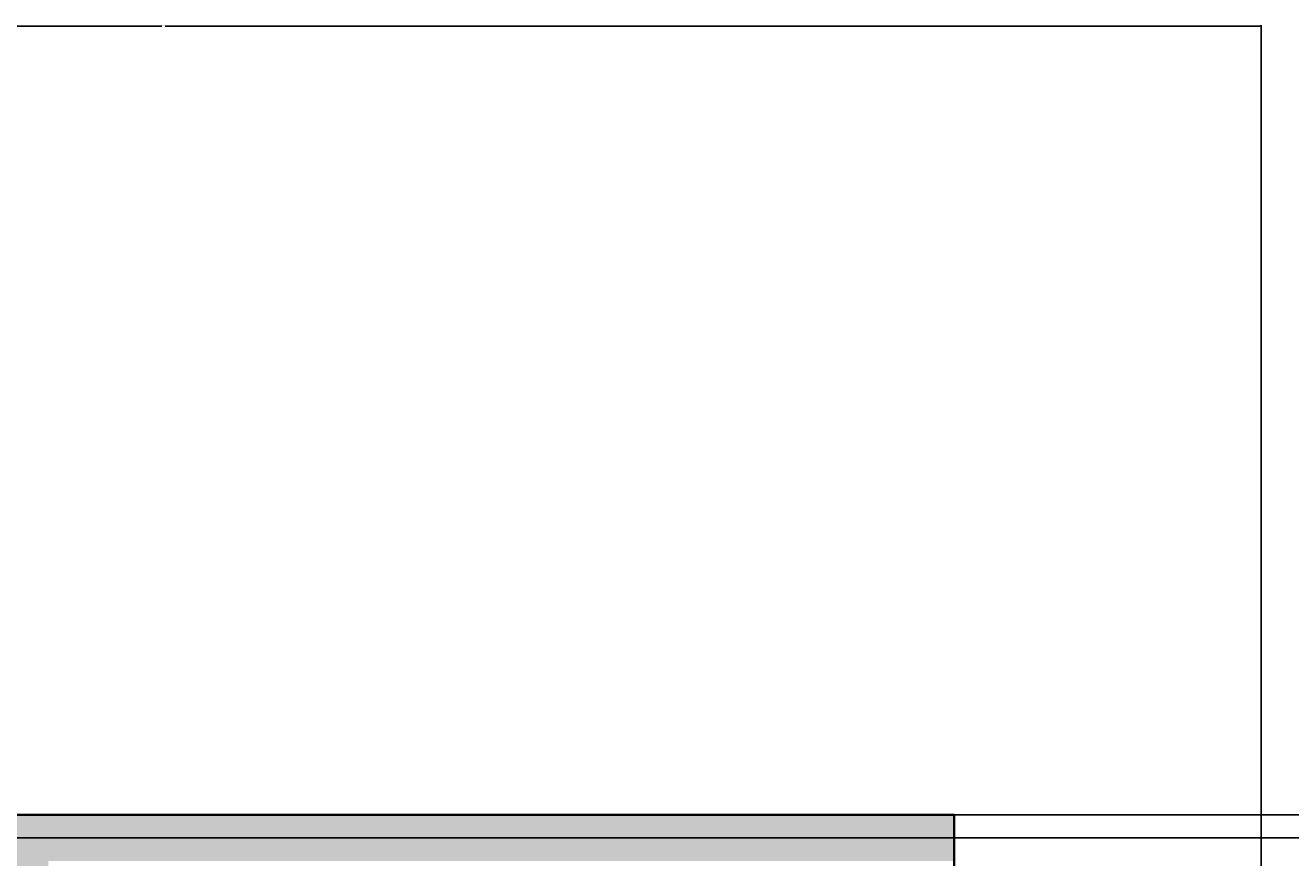
# Model space of a CAD drawing. Units: inches. Extents: x 5716 to 6907, y 12769 to 13594.
# Tile 10 of 17: x 6007 to 6254, y 13432 to 13594. Entities that reach past the tile are written whole.
import ezdxf

# ---------------------------------------------------------------- set-up
doc = ezdxf.new("R2010")
doc.units = ezdxf.units.IN
for name, color, linetype, lineweight in [('A-ANNO-DIMS', 2, 'Continuous', 18), ('A-WALL', 7, 'Continuous', 35), ('A-WALL-PATT', 252, 'Continuous', 13)]:
    doc.layers.add(name, color=color, linetype=linetype, lineweight=lineweight)
doc.styles.get("Standard").update_dxf_attribs({"font": 'arial.ttf'})
doc.dimstyles.get("Standard").update_dxf_attribs({"dimtxt": 0.18, "dimasz": 0.18, "dimexe": 0.18, "dimexo": 0.0625, "dimgap": 0.09, "dimtad": 0, "dimtih": 1, "dimtoh": 1, "dimdec": 4, "dimzin": 0, "dimdsep": 46, "dimtxsty": 'Standard', "dimcen": 0.09, "dimadec": 0, "dimazin": 0, "dimtfac": 1, "dimtdec": 4, "dimtofl": 0, "dimtmove": 0, "dimatfit": 3, "dimfxl": 1, "dimtolj": 1, "dimtzin": 0, "dimarcsym": 0})

# ---------------------------------------------------------------- blocks, each defined once
blk = doc.blocks.new('*D51')
at = {"layer": 'A-ANNO-DIMS', "color": 0, "lineweight": -2, "transparency": 16777216}
for p, q in [((5819.02, 13440.21), (5819.02, 13594.38)), ((5819.2, 13594.2), (6033.23, 13594.2)), ((6247.84, 13594.2), (6033.82, 13594.2)), ((6248.02, 13194.21), (6248.02, 13594.38))]:
    blk.add_line(p, q, dxfattribs=at)
at = {"layer": 'A-ANNO-DIMS', "color": 0, "transparency": 16777216}
for points in [[(5819.2, 13594.23), (5819.2, 13594.17), (5819.02, 13594.2)], [(6247.84, 13594.23), (6247.84, 13594.17), (6248.02, 13594.2)]]:
    blk.add_solid(points, dxfattribs=at)
at = {"layer": 'Defpoints', "color": 0, "transparency": 16777216}
for p in [(6248.02, 13594.2), (5819.02, 13440.15), (6248.02, 13194.15)]:
    blk.add_point(p, dxfattribs=at)
at = {"layer": 'A-ANNO-DIMS', "color": 0, "transparency": 16777216, "insert": (6033.52, 13594.2), "char_height": 0.18, "attachment_point": 5}
blk.add_mtext('\\A1;429', dxfattribs=at)
blk = doc.blocks.new('*D52')
at = {"layer": 'A-ANNO-DIMS', "color": 0, "lineweight": -2, "transparency": 16777216}
for p, q in [((6267.34, 13440.15), (5716.04, 13440.15)), ((5716.22, 13439.97), (5716.22, 13140.83)), ((5716.22, 12841.33), (5716.22, 13140.47)), ((6267.34, 12841.15), (5716.04, 12841.15))]:
    blk.add_line(p, q, dxfattribs=at)
at = {"layer": 'A-ANNO-DIMS', "color": 0, "transparency": 16777216}
for points in [[(5716.19, 13439.97), (5716.25, 13439.97), (5716.22, 13440.15)], [(5716.19, 12841.33), (5716.25, 12841.33), (5716.22, 12841.15)]]:
    blk.add_solid(points, dxfattribs=at)
at = {"layer": 'Defpoints', "color": 0, "transparency": 16777216}
for p in [(6267.41, 13440.15), (5716.22, 12841.15), (6267.41, 12841.15)]:
    blk.add_point(p, dxfattribs=at)
at = {"layer": 'A-ANNO-DIMS', "color": 0, "transparency": 16777216, "insert": (5716.22, 13140.65), "char_height": 0.18, "attachment_point": 5}
blk.add_mtext('\\A1;599', dxfattribs=at)
blk = doc.blocks.new('*D58')
at = {"layer": 'A-ANNO-DIMS', "color": 0, "lineweight": -2, "transparency": 16777216}
for p, q in [((6736.67, 13435.65), (5716.04, 13435.65)), ((5716.22, 13435.47), (5716.22, 13365.33)), ((5716.22, 13294.83), (5716.22, 13364.97)), ((6736.67, 13294.65), (5716.04, 13294.65))]:
    blk.add_line(p, q, dxfattribs=at)
at = {"layer": 'A-ANNO-DIMS', "color": 0, "transparency": 16777216}
for points in [[(5716.19, 13435.47), (5716.25, 13435.47), (5716.22, 13435.65)], [(5716.19, 13294.83), (5716.25, 13294.83), (5716.22, 13294.65)]]:
    blk.add_solid(points, dxfattribs=at)
at = {"layer": 'Defpoints', "color": 0, "transparency": 16777216}
for p in [(6736.73, 13435.65), (5716.22, 13294.65), (6736.73, 13294.65)]:
    blk.add_point(p, dxfattribs=at)
at = {"layer": 'A-ANNO-DIMS', "color": 0, "transparency": 16777216, "insert": (5716.22, 13365.15), "char_height": 0.18, "attachment_point": 5}
blk.add_mtext('\\A1;141', dxfattribs=at)

msp = doc.modelspace()

# ---------------------------------------------------------------- hatches: boundary and pattern name
at = {"layer": 'A-WALL-PATT'}
h = msp.add_hatch(color=256, dxfattribs=at)
h.dxf.hatch_style = 1
h.paths.add_polyline_path([(6188.02, 13440.15), (5819.02, 13440.15), (5819.02, 13431.15), (6002.02, 13431.15), (6002.02, 13290.15), (6011.02, 13290.15), (6011.02, 13431.15), (6188.02, 13431.15)])

# ---------------------------------------------------------------- linework, layer by layer
at = {"layer": 'A-WALL'}
for p, q in [((5819.02, 13440.15), (6188.02, 13440.15)), ((6188.02, 13440.15), (6188.02, 13185.15))]:
    msp.add_line(p, q, dxfattribs=at)

# ---------------------------------------------------------------- dimensions: what is measured, and where the dimension line sits
at = {"layer": 'A-ANNO-DIMS'}
dim = msp.add_linear_dim(base=(6248.02, 13594.2), p1=(5819.02, 13440.15), p2=(6248.02, 13194.15), dimstyle='Standard', override={"dimdec": 0, "dimlfac": 1, "dimrnd": 0, "dimzin": 0, "dimdsep": 46, "dimlunit": 2}, dxfattribs=at)
dim.commit()
dim.dimension.update_dxf_attribs({"geometry": '*D51', "text_midpoint": (6033.52, 13594.2)})
for base, p1, p2, picture, middle in [((5716.22, 12841.15), (6267.41, 13440.15), (6267.41, 12841.15), '*D52', (5716.22, 13140.65)), ((5716.22, 13294.65), (6736.73, 13435.65), (6736.73, 13294.65), '*D58', (5716.22, 13365.15))]:
    dim = msp.add_linear_dim(base=base, p1=p1, p2=p2, angle=90, dimstyle='Standard', override={"dimdec": 0, "dimlfac": 1, "dimrnd": 0, "dimzin": 0, "dimdsep": 46, "dimlunit": 2}, dxfattribs=at)
    dim.commit()
    dim.dimension.update_dxf_attribs({"geometry": picture, "text_midpoint": middle})

doc.saveas('drawing.dxf')
